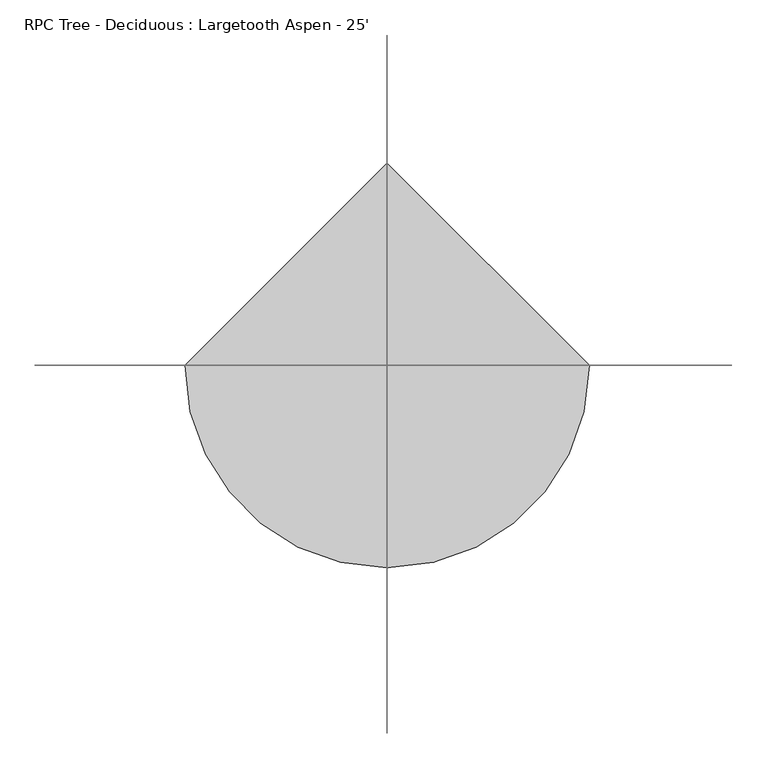
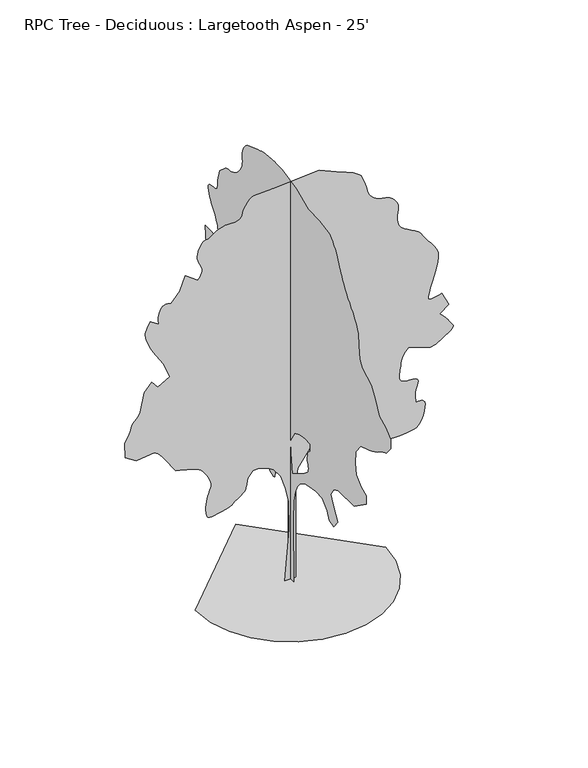
"""IFC4 building model written with IfcOpenShell, lengths in millimetres: geographic element geometry, RPC Tree - Deciduous : Largetooth Aspen - 25'."""

from ifc_helpers import new_model, si_unit, origin, place, context, project, spatial, triangles, source, transform, mapped, element, save


def rpc_tree_deciduous_largetooth_aspen_25_807f66b4(model_context):
    return source(origin(), model_context, "Body", "Tessellation", [
        triangles([(26.0697205, 0.000114, 0.0015477), (-29.1730399, 0.000114, 0.0015477), (-6.4261123, 9.81e-05, 266.4664568), (-9.6756528, 8.92e-05, 415.9470311), (-25.9234267, 8.45e-05, 493.9371471), (-48.6706393, 8.05e-05, 562.1781489), (-84.4157958, 7.76e-05, 610.9215763), (-113.6617395, 7.66e-05, 627.1696398), (-159.1557286, 7.56e-05, 643.4177032), (-191.6518556, 7.56e-05, 643.4177032), (-214.3988501, 7.76e-05, 610.9215763), (-224.1479643, 8.01e-05, 568.6770982), (-224.9530387, 8.04e-05, 563.7605742), (-226.4124337, 8.07e-05, 558.5873071), (-229.1782896, 8.1e-05, 552.903388), (-233.9063258, 8.14e-05, 546.4513836), (-241.248047, 8.18e-05, 538.9766945), (-251.8591362, 8.24e-05, 530.2225413), (-266.392497, 8.3e-05, 519.9336345), (-280.2623081, 8.36e-05, 510.0998597), (-289.8115798, 8.4e-05, 502.539093), (-297.0878617, 8.44e-05, 496.7414091), (-304.1365594, 8.46e-05, 492.1940123), (-313.003787, 8.49e-05, 488.3855238), (-325.7370941, 8.51e-05, 484.8039474), (-344.3818863, 8.53e-05, 480.9385583), (-364.9121012, 8.56e-05, 476.5525978), (-382.0882693, 8.58e-05, 472.5065875), (-396.1379931, 8.6e-05, 469.9398474), (-407.2889113, 8.6e-05, 469.9867922), (-415.7685173, 8.57e-05, 473.7860152), (-421.803069, 8.52e-05, 482.4733483), (-425.6214769, 8.43e-05, 497.1866218), (-427.2885263, 8.33e-05, 514.7041572), (-427.0232446, 8.23e-05, 531.0845163), (-425.2801097, 8.14e-05, 546.3852539), (-422.5135271, 8.05e-05, 560.6625801), (-419.1787379, 7.98e-05, 573.9733955), (-415.7301112, 7.9e-05, 586.3745645), (-412.6228881, 7.83e-05, 597.9237505), (-409.3641844, 7.77e-05, 608.0227707), (-405.6503122, 7.72e-05, 616.6439014), (-402.2209067, 7.67e-05, 624.6968256), (-399.8141859, 7.62e-05, 633.0910807), (-399.1698575, 7.57e-05, 642.7356955), (-401.0267936, 7.5e-05, 654.5402075), (-406.1239388, 7.41e-05, 669.4142269), (-413.6370704, 7.31e-05, 685.5008177), (-422.0590854, 7.22e-05, 700.2233202), (-431.1069706, 7.14e-05, 713.4111053), (-440.4954964, 7.08e-05, 724.8969595), (-449.9409591, 7.02e-05, 734.4981903), (-459.1587831, 6.97e-05, 742.058194), (-467.8659914, 6.94e-05, 747.406414), (-477.7374455, 6.92e-05, 751.5811592), (-490.3384933, 6.89e-05, 755.763026), (-505.2125127, 6.87e-05, 759.9377712), (-521.9057888, 6.84e-05, 764.1196381), (-539.9631168, 6.82e-05, 768.2943832), (-558.9300914, 6.79e-05, 772.4691284), (-578.351544, 6.77e-05, 776.6509953), (-633.5939569, 6.28e-05, 857.8912399), (-646.194932, 6.18e-05, 874.9245026), (-656.4077534, 6.11e-05, 887.526931), (-664.6306526, 6.05e-05, 896.4311113), (-671.2625879, 6.02e-05, 902.3767513), (-676.7004101, 6e-05, 906.110535), (-681.3431499, 5.98e-05, 908.3650486), (-685.5875856, 5.97e-05, 909.8799271), (-776.5727297, 6.03e-05, 900.1364811), (-831.8187035, 5.82e-05, 935.8813923), (-835.0688684, 5.37e-05, 1010.621307), (-828.8316765, 5.31e-05, 1021.7515869), (-822.8006493, 5.24e-05, 1032.8249662), (-817.1608772, 5.18e-05, 1043.791666), (-812.1184525, 5.11e-05, 1054.5805424), (-807.879685, 5.05e-05, 1065.1418163), (-804.62952, 4.99e-05, 1075.41866), (-802.5741949, 4.93e-05, 1085.3612217), (-799.3666872, 4.87e-05, 1094.7561424), (-793.2717104, 4.82e-05, 1103.6461521), (-785.3489382, 4.77e-05, 1112.3014378), (-776.6865309, 4.71e-05, 1121.0207457), (-768.3725761, 4.66e-05, 1130.0743355), (-761.473942, 4.6e-05, 1139.7608809), (-757.0787888, 4.54e-05, 1150.3506414), (-737.5776535, 3.96e-05, 1247.8418564), (-698.5861382, 3.71e-05, 1290.0799759), (-669.3395222, 3.92e-05, 1254.3350647), (-607.5974696, 3.73e-05, 1286.8368599), (-640.0935602, 3.24e-05, 1368.0701283), (-692.0865349, 2.76e-05, 1449.3103729), (-698.3393509, 2.69e-05, 1460.8602493), (-705.5018497, 2.6e-05, 1475.2548649), (-712.891951, 2.51e-05, 1491.3493767), (-719.8261208, 2.41e-05, 1508.0127491), (-725.6224239, 2.31e-05, 1524.1071156), (-729.6051023, 2.23e-05, 1538.5018764), (-731.0844452, 2.16e-05, 1550.0517529), (-730.3234451, 2.1e-05, 1559.7027626), (-728.2040977, 2.04e-05, 1569.1901196), (-724.9396894, 1.99e-05, 1578.5282124), (-720.7720659, 1.93e-05, 1587.7523586), (-715.9216352, 1.88e-05, 1596.8984573), (-710.6175259, 1.82e-05, 1605.9804611), (-705.0850874, 1.77e-05, 1615.0410999), (-662.8405729, 1.94e-05, 1585.796664), (-664.186203, 1.89e-05, 1594.8715462), (-665.2472574, 1.84e-05, 1604.0887161), (-665.7394512, 1.78e-05, 1613.5903164), (-665.3795895, 1.72e-05, 1623.5186348), (-663.8825151, 1.66e-05, 1634.0159592), (-660.964452, 1.59e-05, 1645.224432), (-656.3416237, 1.52e-05, 1657.2863411), (-650.2971525, 1.46e-05, 1667.8335171), (-643.3999718, 1.41e-05, 1674.7960281), (-635.7922239, 1.39e-05, 1678.7716576), (-627.6162695, 1.38e-05, 1680.3647289), (-619.0136696, 1.38e-05, 1680.1656132), (-610.1272207, 1.39e-05, 1678.7716576), (-601.0985204, 1.4e-05, 1676.7803547), (-558.8540059, 1.11e-05, 1725.5259258), (-529.6080803, 6.9e-06, 1797.0157482), (-467.8659914, 9.6e-06, 1751.5202694), (-461.6700397, 9.1e-06, 1759.8911247), (-455.9000793, 8.6e-06, 1768.3116863), (-450.982865, 8.1e-06, 1776.8460491), (-447.3450783, 7.5e-06, 1785.5511864), (-445.4127471, 7e-06, 1794.4909023), (-445.6111725, 6.5e-06, 1803.7080723), (-448.3684896, 5.9e-06, 1813.2666458), (-452.8589859, 5.3e-06, 1823.0455547), (-457.6339851, 4.7e-06, 1832.9881165), (-462.181382, 4.1e-06, 1843.2792034), (-465.9898705, 3.5e-06, 1854.0823231), (-468.5480355, 2.8e-06, 1865.5611282), (-469.3438808, 2e-06, 1877.8932243), (-467.8659914, 1.2e-06, 1891.2566528), (-464.322821, 4e-07, 1904.904657), (-459.4148357, -3e-07, 1917.7062012), (-453.3703282, -1e-06, 1929.1992496), (-446.4169373, -1.6e-06, 1938.9284523), (-438.7808118, -2e-06, 1946.4386044), (-430.6894815, -2.3e-06, 1951.2819134), (-422.3720023, -2.4e-06, 1952.9959076), (-413.0588717, -2.6e-06, 1955.3357357), (-401.9840753, -2.9e-06, 1961.3738846), (-389.3737985, -3.4e-06, 1969.6238171), (-375.456334, -4e-06, 1978.6133846), (-360.4592843, -4.5e-06, 1986.8631718), (-344.6094887, -4.8e-06, 1992.9013206), (-328.1338228, -5e-06, 1995.2411488), (-311.3459667, -5e-06, 1995.1487125), (-294.899496, -5e-06, 1995.276757), (-279.5326106, -5e-06, 1996.2652142), (-265.9849819, -5.2e-06, 1998.7259651), (-254.9948097, -5.4e-06, 2003.2919655), (-247.3017654, -5.9e-06, 2010.5889038), (-243.6447939, -6.5e-06, 2021.2354923), (-240.5752501, -7.3e-06, 2034.9474461), (-234.6068645, -8.2e-06, 2050.1315483), (-226.4216809, -9.1e-06, 2065.4934013), (-216.7009988, -1e-05, 2079.7102661), (-206.1283157, -1.07e-05, 2091.4877449), (-195.3849308, -1.12e-05, 2099.510075), (-185.1529063, -1.13e-05, 2102.475737), (-90.9154535, -1.17e-05, 2108.9762123), (143.0548945, -1.27e-05, 2125.2271099), (260.03936, -9.6e-06, 2073.2313011), (279.432326, -9.1e-06, 2065.5361313), (298.2008752, -8.7e-06, 2057.648822), (315.7177202, -8.2e-06, 2049.3563049), (331.359825, -7.7e-06, 2040.4734169), (344.499975, -7.1e-06, 2030.7869442), (354.5136443, -6.4e-06, 2020.1117237), (360.7764524, -5.7e-06, 2008.2418087), (364.9448027, -5e-06, 1996.5852528), (369.0562523, -4.4e-06, 1986.2444595), (373.0545911, -3.8e-06, 1976.5223785), (376.8823008, -3.3e-06, 1966.7434696), (380.4823717, -2.6e-06, 1956.2247803), (383.797976, -1.9e-06, 1944.2907703), (386.7729398, -1.1e-06, 1930.2518017), (391.2164912, -2e-07, 1915.7361179), (398.4451198, 5e-07, 1902.8706242), (407.6629801, 1.2e-06, 1891.7118576), (418.0749536, 1.8e-06, 1882.3098152), (428.8844682, 2.2e-06, 1874.7355682), (439.2964053, 2.6e-06, 1869.0317013), (448.5149923, 2.8e-06, 1865.2553329), (457.0415431, 2.9e-06, 1862.9936977), (465.7950059, 3e-06, 1861.4716976), (474.6060596, 3.1e-06, 1860.2271515), (483.3033122, 3.2e-06, 1858.8189526), (491.7160618, 3.3e-06, 1856.7777981), (499.674406, 3.5e-06, 1853.6627266), (507.0068436, 3.8e-06, 1849.0114117), (514.1032127, 4.1e-06, 1842.6889778), (521.1988552, 4.6e-06, 1835.0648792), (527.8969202, 5.1e-06, 1826.4167152), (533.7991762, 5.7e-06, 1817.0287708), (538.5080094, 6.3e-06, 1807.1859123), (541.6251884, 6.8e-06, 1797.172134), (542.7524451, 7.4e-06, 1787.2651806), (541.7674398, 8.1e-06, 1775.6939392), (539.645222, 9e-06, 1761.1000626), (537.6368053, 1e-05, 1744.4651768), (536.9924406, 1.1e-05, 1726.7492523), (538.9631779, 1.21e-05, 1708.9193813), (544.7992679, 1.31e-05, 1691.943092), (555.751034, 1.4e-05, 1676.7803547), (571.0795315, 1.48e-05, 1664.08549), (588.4548154, 1.54e-05, 1653.2111538), (606.7397458, 1.6e-05, 1643.1903992), (624.7971102, 1.66e-05, 1633.0487217), (641.49035, 1.73e-05, 1621.8331272), (655.6823616, 1.81e-05, 1608.5692566), (666.2365866, 1.91e-05, 1592.296994), (677.0367994, 2.01e-05, 1574.1543514), (691.3610704, 2.12e-05, 1555.7839611), (707.1639576, 2.24e-05, 1536.9585114), (722.4006729, 2.35e-05, 1517.4503998), (735.0173447, 2.47e-05, 1497.0318787), (742.9756525, 2.6e-05, 1475.4824673), (744.227393, 2.74e-05, 1452.5606106), (739.640173, 2.9e-05, 1426.0825756), (732.2152628, 3.08e-05, 1395.5081337), (723.0834074, 3.27e-05, 1363.1201397), (713.3755697, 3.46e-05, 1331.1802288), (704.2458944, 3.64e-05, 1301.9712559), (696.8181501, 3.78e-05, 1277.7690994), (692.2330376, 3.88e-05, 1260.8353947), (692.0054352, 3.94e-05, 1250.6723522), (696.3828569, 3.98e-05, 1244.7695148), (704.5965271, 3.99e-05, 1242.4224197), (715.878978, 3.99e-05, 1242.9132328), (729.4628872, 3.97e-05, 1245.5374912), (744.5829672, 3.95e-05, 1249.5841919), (760.4711689, 3.92e-05, 1254.3350647), (796.2160801, 4.35e-05, 1182.845315), (750.7277229, 4.56e-05, 1147.1004765), (757.676136, 4.6e-05, 1140.8134329), (764.5747702, 4.64e-05, 1134.3771252), (771.3596031, 4.68e-05, 1127.6633635), (777.973807, 4.72e-05, 1120.5158346), (784.3603357, 4.76e-05, 1112.8064215), (790.4624342, 4.81e-05, 1104.3857872), (796.2160801, 4.87e-05, 1095.1117893), (802.3750065, 4.92e-05, 1086.0795645), (808.8754091, 4.97e-05, 1078.1852062), (814.4654022, 5.01e-05, 1070.9807768), (817.8933907, 5.05e-05, 1063.9968281), (817.9147556, 5.1e-05, 1056.785277), (813.270635, 5.14e-05, 1048.8980404), (802.7164101, 5.2e-05, 1039.8658155), (731.2266603, 5.49e-05, 991.1202444), (701.9814251, 5.51e-05, 987.8700068), (594.7461102, 5.3e-05, 1023.6149179), (587.1284429, 5.34e-05, 1015.9055048), (579.7675186, 5.39e-05, 1007.8831747), (572.917973, 5.44e-05, 999.2350107), (566.8350958, 5.5e-05, 989.6409016), (561.7763203, 5.56e-05, 978.8093679), (557.9962821, 5.64e-05, 966.4060553), (555.751034, 5.72e-05, 952.1251682), (554.18783, 5.8e-05, 938.2638777), (552.3970236, 5.87e-05, 926.7922668), (550.5493166, 5.93e-05, 916.9136547), (548.8154108, 5.99e-05, 907.8245293), (547.366008, 6.04e-05, 898.7425255), (546.3710469, 6.1e-05, 888.8568644), (546.0019197, 6.17e-05, 877.3852535), (548.5217151, 6.23e-05, 866.5607689), (555.0213547, 6.28e-05, 858.8015768), (563.9077672, 6.31e-05, 853.5956446), (573.5900614, 6.33e-05, 850.4449648), (582.4764739, 6.34e-05, 848.8234795), (588.9761498, 6.34e-05, 848.2260595), (591.4959088, 6.34e-05, 848.140745), (595.0490713, 6.34e-05, 848.3896397), (604.0016499, 6.34e-05, 848.5176115), (615.7968601, 6.34e-05, 847.6286396), (627.8765734, 6.36e-05, 844.8051928), (637.6819342, 6.4e-05, 839.1440557), (642.6560492, 6.45e-05, 829.7206484), (640.2400629, 6.54e-05, 815.6459988), (634.4132383, 6.63e-05, 799.5017807), (630.6332365, 6.72e-05, 784.3817007), (628.5579271, 6.81e-05, 770.115057), (627.8474327, 6.89e-05, 756.5240261), (628.1603497, 6.97e-05, 743.4521496), (629.1553471, 7.04e-05, 730.7216766), (630.4909487, 7.12e-05, 718.1547838), (641.5372948, 7.11e-05, 719.3994026), (652.016161, 7.11e-05, 719.7336845), (661.3570152, 7.12e-05, 718.2401711), (668.993177, 7.14e-05, 714.0298903), (674.3556404, 7.19e-05, 706.1732477), (676.8753994, 7.26e-05, 693.7720425), (675.9849741, 7.37e-05, 675.9131035), (672.4133171, 7.49e-05, 655.5067183), (667.3069427, 7.6e-05, 636.4067213), (660.7226063, 7.71e-05, 619.1267441), (652.7166269, 7.8e-05, 604.1766028), (643.347286, 7.87e-05, 592.0684393), (632.6701035, 7.92e-05, 583.3149765), (620.7425611, 7.95e-05, 578.4262124), (609.5532732, 7.96e-05, 576.0102625), (600.0701311, 7.97e-05, 574.2194561), (590.8138647, 7.98e-05, 572.8838181), (580.3073112, 7.99e-05, 571.8319565), (567.0718909, 7.99e-05, 570.8945864), (549.630441, 8e-05, 569.8996253), (526.5043817, 8.01e-05, 568.6770982), (501.3699057, 8e-05, 569.0845951), (478.622893, 7.98e-05, 572.7323376), (457.865112, 7.95e-05, 579.0798062), (438.6997121, 7.89e-05, 587.5871721), (420.7277349, 7.83e-05, 597.7153693), (403.5515305, 7.77e-05, 608.9231518), (386.7729398, 7.7e-05, 620.6707632), (315.281773, 7.29e-05, 688.9117287), (240.541822, 7.1e-05, 721.4050215), (152.8033002, 7.14e-05, 714.9117405), (110.5587767, 7.33e-05, 682.4127794), (81.3128329, 7.58e-05, 640.168265), (35.8184146, 7.97e-05, 575.1767378), (26.0697205, 8.45e-05, 493.9371471), (26.0697205, 9.5e-05, 318.4601037), (-0.0006638, 25.4362563, 3.1e-06), (-0.0006638, -26.5568933, 0.0), (-0.0006638, -23.3073528, 324.9576359), (-0.0006638, -26.5568933, 428.9442029), (-0.0006638, -39.5552709, 484.1866158), (-0.0006638, -59.0527272, 526.4311303), (-0.0006638, -85.049478, 558.9272573), (-0.0006638, -124.044536, 581.67427), (-0.0006638, -156.5399363, 588.1731829), (-0.0006638, -221.5314634, 601.1717717), (-0.0006638, -276.7745849, 597.9222971), (-0.0006638, -319.0191175, 555.6777826), (-0.0006638, -338.5166556, 516.6827428), (-0.0006638, -374.2615305, 503.6841539), (-0.0006638, -413.2565703, 552.4276176), (-0.0006638, -371.0120559, 617.4198715), (-0.0006638, -351.5145178, 662.9138243), (-0.0006638, -374.2615305, 701.9081738), (-0.0006638, -416.506045, 721.4050215), (-0.0006638, -552.9880122, 721.4050215), (-0.0006638, -660.2240902, 796.1449362), (-0.0006638, -660.2240902, 841.6403423), (-0.0006638, -614.7300648, 861.1343559), (-0.0006638, -572.4855503, 900.1293594), (-0.0006638, -562.7371628, 955.3753332), (-0.0006638, -569.2360757, 1020.364753), (-0.0006638, -611.4806265, 1075.6107267), (-0.0006638, -686.2205412, 1101.6049976), (-0.0006638, -698.7362017, 1106.4980856), (-0.0006638, -711.1374069, 1111.4693665), (-0.0006638, -723.3110098, 1116.6113491), (-0.0006638, -735.1453892, 1122.0164698), (-0.0006638, -746.5245638, 1127.7557997), (-0.0006638, -757.3348051, 1133.9219204), (-0.0006638, -767.4622393, 1140.6000738), (-0.0006638, -777.2056852, 1147.185791), (-0.0006638, -786.9562529, 1153.0887737), (-0.0006638, -796.7067478, 1158.4227505), (-0.0006638, -806.4573154, 1163.3015951), (-0.0006638, -816.2007614, 1167.8390362), (-0.0006638, -825.951329, 1172.1488749), (-0.0006638, -835.701824, 1176.344985), (-0.0006638, -871.4467352, 1221.8403912), (-0.0006638, -871.4467352, 1267.3357246), (-0.0006638, -829.201494, 1306.3308735), (-0.0006638, -773.9626419, 1335.5753094), (-0.0006638, -738.2106091, 1403.8148941), (-0.0006638, -702.4693314, 1455.8107029), (-0.0006638, -624.479179, 1498.0559441), (-0.0006638, -601.7322026, 1533.8008553), (-0.0006638, -595.232563, 1605.2905323), (-0.0006638, -588.7336138, 1663.7795494), (-0.0006638, -581.7610016, 1678.3663044), (-0.0006638, -574.7315251, 1692.6898487), (-0.0006638, -567.5875208, 1706.5013603), (-0.0006638, -560.2735414, 1719.5447502), (-0.0006638, -552.7327226, 1731.5711964), (-0.0006638, -544.9066741, 1742.3102211), (-0.0006638, -536.7406754, 1751.5202694), (-0.0006638, -526.6124783, 1762.4087036), (-0.0006638, -513.8137319, 1777.3297405), (-0.0006638, -499.6495165, 1794.754113), (-0.0006638, -485.4297812, 1813.1386013), (-0.0006638, -472.4596427, 1830.9612053), (-0.0006638, -462.0476692, 1846.6787052), (-0.0006638, -455.5010848, 1858.7548576), (-0.0006638, -450.7737571, 1868.9036568), (-0.0006638, -445.1367828, 1879.8490643), (-0.0006638, -438.8739747, 1891.5838131), (-0.0006638, -432.2711801, 1904.1222919), (-0.0006638, -425.6108308, 1917.4501122), (-0.0006638, -419.1780112, 1931.5745407), (-0.0006638, -413.2565703, 1946.4955776), (-0.0006638, -406.7384362, 1961.4378342), (-0.0006638, -398.5148466, 1975.6974289), (-0.0006638, -388.8702682, 1989.3880177), (-0.0006638, -378.0892038, 2002.6234016), (-0.0006638, -366.4546669, 2015.517382), (-0.0006638, -354.2526501, 2028.1839054), (-0.0006638, -341.7660939, 2040.7366276), (-0.0006638, -250.7774072, 2056.9804035), (-0.0006638, -153.2904798, 2060.2304958), (-0.0006638, -49.3039627, 2105.7259747), (-0.0006638, 74.1795065, 2131.7203182), (-0.0006638, 90.8727781, 2132.40298), (-0.0006638, 107.452253, 2133.0004726), (-0.0006638, 123.8048613, 2133.4271908), (-0.0006638, 139.8153757, 2133.5978199), (-0.0006638, 155.3721478, 2133.4271908), (-0.0006638, 170.3599684, 2132.8298435), (-0.0006638, 184.6657449, 2131.7203182), (-0.0006638, 198.4217548, 2130.297876), (-0.0006638, 211.9501987, 2128.7119263), (-0.0006638, 225.4224323, 2126.7774513), (-0.0006638, 239.0084853, 2124.3309437), (-0.0006638, 252.8782783, 2121.2087505), (-0.0006638, 267.2025493, 2117.2259995), (-0.0006638, 282.1526723, 2112.2263046), (-0.0006638, 376.3908337, 2079.7316311), (-0.0006638, 384.7090396, 2072.7121468), (-0.0006638, 392.7996431, 2065.3441372), (-0.0006638, 400.4357686, 2057.3004421), (-0.0006638, 407.3891596, 2048.239658), (-0.0006638, 413.4336671, 2037.8064285), (-0.0006638, 418.3416524, 2025.6733028), (-0.0006638, 421.8848228, 2011.4849247), (-0.0006638, 423.1066958, 1997.9295021), (-0.0006638, 422.1116984, 1986.9912163), (-0.0006638, 420.2647182, 1977.2976219), (-0.0006638, 418.9283898, 1967.4902264), (-0.0006638, 419.4689092, 1956.210537), (-0.0006638, 423.248911, 1942.0789867), (-0.0006638, 431.6332466, 1923.7514717), (-0.0006638, 443.1155763, 1905.1322594), (-0.0006638, 455.053038, 1890.609454), (-0.0006638, 467.1036106, 1879.4934174), (-0.0006638, 478.9273075, 1871.1084641), (-0.0006638, 490.1827251, 1864.7716415), (-0.0006638, 500.5278422, 1859.8004333), (-0.0006638, 509.6233626, 1855.5047653), (-0.0006638, 517.979248, 1852.3896938), (-0.0006638, 526.3351333, 1850.8676937), (-0.0006638, 534.6910186, 1850.1351803), (-0.0006638, 543.0475943, 1849.4097885), (-0.0006638, 551.4034796, 1847.8806667), (-0.0006638, 559.7593649, 1844.7655952), (-0.0006638, 568.1152502, 1839.2609894), (-0.0006638, 616.8594406, 1797.0157482), (-0.0006638, 636.3562157, 1735.2764935), (-0.0006638, 635.7218067, 1725.5615341), (-0.0006638, 635.4565613, 1716.0811535), (-0.0006638, 635.9302242, 1707.0490013), (-0.0006638, 637.5126131, 1698.7066326), (-0.0006638, 640.5722374, 1691.2674065), (-0.0006638, 645.4802227, 1684.9661922), (-0.0006638, 652.6042791, 1680.0305923), (-0.0006638, 662.5141394, 1677.2070728), (-0.0006638, 674.5838968, 1676.1473991), (-0.0006638, 687.3926353, 1675.429129), (-0.0006638, 699.5199474, 1673.6296749), (-0.0006638, 709.5428822, 1669.3270306), (-0.0006638, 716.0425581, 1661.0984631), (-0.0006638, 717.5929722, 1647.5357735), (-0.0006638, 715.1606352, 1631.7685673), (-0.0006638, 710.8507965, 1617.7080883), (-0.0006638, 704.9763004, 1605.0700516), (-0.0006638, 697.852244, 1593.5700268), (-0.0006638, 689.7900908, 1582.9234383), (-0.0006638, 681.1020309, 1572.8457104), (-0.0006638, 672.1018536, 1563.0452911), (-0.0006638, 665.1668844, 1551.2109844), (-0.0006638, 658.4026897, 1539.4121407), (-0.0006638, 651.9791719, 1527.6631485), (-0.0006638, 646.0676868, 1515.9994709), (-0.0006638, 640.8374828, 1504.4495945), (-0.0006638, 636.4607878, 1493.0420059), (-0.0006638, 633.1067774, 1481.8050465), (-0.0006638, 631.3636425, 1471.2366508), (-0.0006638, 631.4966286, 1461.685199), (-0.0006638, 633.1920919, 1452.9873287), (-0.0006638, 636.1385691, 1444.9719749), (-0.0006638, 640.023143, 1437.4689445), (-0.0006638, 644.5328968, 1430.3071724), (-0.0006638, 649.3548409, 1423.3160294), (-0.0006638, 691.5993553, 1429.8163593), (-0.0006638, 743.5944374, 1429.8163593), (-0.0006638, 737.0940348, 1335.5753094), (-0.0006638, 678.6007301, 1234.8410511), (-0.0006638, 676.5076893, 1223.013866), (-0.0006638, 674.3855078, 1211.2790445), (-0.0006638, 672.206353, 1199.7078758), (-0.0006638, 669.9418837, 1188.3997725), (-0.0006638, 667.5636858, 1177.425951), (-0.0006638, 665.0438541, 1166.8789204), (-0.0006638, 662.3533934, 1156.8509714), (-0.0006638, 658.3266043, 1146.0123161), (-0.0006638, 652.4243483, 1133.4098877), (-0.0006638, 645.5555815, 1119.676569), (-0.0006638, 638.6306408, 1105.4241686), (-0.0006638, 632.557683, 1091.2926184), (-0.0006638, 628.2471176, 1077.8936543), (-0.0006638, 626.6078281, 1065.8601591), (-0.0006638, 627.9342007, 1055.1921329), (-0.0006638, 631.6480728, 1045.3776157), (-0.0006638, 637.3512131, 1036.274247), (-0.0006638, 644.6459713, 1027.7398842), (-0.0006638, 653.1348427, 1019.6251179), (-0.0006638, 662.419523, 1011.8019035), (-0.0006638, 672.1018536, 1004.1209044), (-0.0006638, 759.8382133, 1023.6149179), (-0.0006638, 764.6814497, 1009.7109701), (-0.0006638, 769.325643, 995.9137018), (-0.0006638, 773.5714594, 982.3511576), (-0.0006638, 777.2128069, 969.1228226), (-0.0006638, 780.0647404, 956.3496923), (-0.0006638, 781.9209497, 944.1454954), (-0.0006638, 782.5894409, 932.6311546), (-0.0006638, 778.8201216, 921.6574059), (-0.0006638, 769.1335762, 910.9111868), (-0.0006638, 755.9835068, 900.2289173), (-0.0006638, 741.8092993, 889.4257977), (-0.0006638, 729.057534, 878.3453693), (-0.0006638, 720.174646, 866.8026146), (-0.0006638, 717.5929722, 854.6410749), (-0.0006638, 719.9328003, 842.956105), (-0.0006638, 723.9795736, 832.8072332), (-0.0006638, 729.4486439, 823.9457102), (-0.0006638, 736.0486044, 816.1012035), (-0.0006638, 743.5090502, 809.0247459), (-0.0006638, 751.5313803, 802.4532721), (-0.0006638, 759.8382133, 796.1449362), (-0.0006638, 779.3392759, 731.1555164), (-0.0006638, 760.6276274, 730.5083176), (-0.0006638, 742.4564981, 730.18123), (-0.0006638, 725.3664076, 730.4727819), (-0.0006638, 709.8935148, 731.7031574), (-0.0006638, 696.5826994, 734.1852734), (-0.0006638, 685.9716465, 738.231974), (-0.0006638, 678.6007301, 744.156249), (-0.0006638, 671.5143894, 751.4958447), (-0.0006638, 661.6997995, 759.5181747), (-0.0006638, 649.6108572, 768.1094381), (-0.0006638, 635.7026218, 777.163028), (-0.0006638, 620.4303709, 786.550827), (-0.0006638, 604.2491275, 796.1663012), (-0.0006638, 587.612752, 805.8955038), (-0.0006638, 586.9214787, 795.4337151), (-0.0006638, 586.2579291, 784.8937334), (-0.0006638, 585.6520068, 774.176001), (-0.0006638, 585.1306724, 763.2021795), (-0.0006638, 584.7231754, 751.8940762), (-0.0006638, 584.4578937, 740.1522057), (-0.0006638, 584.3633137, 727.9053514), (-0.0006638, 583.918101, 715.1464645), (-0.0006638, 582.3925764, 702.6094391), (-0.0006638, 579.5029635, 691.3262615), (-0.0006638, 574.9647958, 682.3160557), (-0.0006638, 568.4942968, 676.6036863), (-0.0006638, 559.8070001, 675.2104574), (-0.0006638, 548.6177121, 679.161161), (-0.0006638, 535.9889408, 686.5035908), (-0.0006638, 523.1901944, 694.528101), (-0.0006638, 510.2485062, 703.1207451), (-0.0006638, 497.1930167, 712.1664865), (-0.0006638, 484.0529031, 721.5543583), (-0.0006638, 470.8558888, 731.1768814), (-0.0006638, 457.6297339, 740.9060841), (-0.0006638, 379.6403083, 763.6502626), (-0.0006638, 301.6501923, 737.6559191), (-0.0006638, 252.9067286, 679.161161), (-0.0006638, 259.1880494, 670.8429914), (-0.0006638, 265.5547029, 662.7524242), (-0.0006638, 272.0913315, 655.1162624), (-0.0006638, 278.8839947, 648.1628351), (-0.0006638, 286.0180432, 642.118364), (-0.0006638, 293.5780832, 637.2103786), (-0.0006638, 301.6501923, 633.6672083), (-0.0006638, 309.3432547, 630.2185816), (-0.0006638, 315.8421676, 625.5765684), (-0.0006638, 321.3468461, 619.9396305), (-0.0006638, 326.054989, 613.506811), (-0.0006638, 330.1671653, 606.4773345), (-0.0006638, 333.8810374, 599.0495539), (-0.0006638, 337.3957938, 591.4226575), (-0.0006638, 328.3194583, 589.3196609), (-0.0006638, 319.101598, 587.131277), (-0.0006638, 309.5985806, 584.7722277), (-0.0006638, 299.6702259, 582.157162), (-0.0006638, 289.1729197, 579.2014194), (-0.0006638, 277.9651372, 575.8189588), (-0.0006638, 265.9046089, 571.9251194), (-0.0006638, 253.8448072, 567.1792972), (-0.0006638, 242.6370247, 561.4093369), (-0.0006638, 232.1397185, 554.7873573), (-0.0006638, 222.2106553, 547.4826433), (-0.0006638, 212.7083283, 539.6665506), (-0.0006638, 203.490468, 531.5090907), (-0.0006638, 194.4141506, 523.1816557), (-0.0006638, 194.4141506, 477.6876666), (-0.0006638, 182.6473543, 470.1560769), (-0.0006638, 171.3072762, 463.3911555), (-0.0006638, 160.8192354, 458.1616782), (-0.0006638, 151.6106223, 455.234386), (-0.0006638, 144.1074647, 455.3766375), (-0.0006638, 138.7357814, 459.3557914), (-0.0006638, 135.9215636, 467.9392791), (-0.0006638, 134.5482372, 477.6684817), (-0.0006638, 133.2879943, 485.2953781), (-0.0006638, 132.2553266, 491.8988631), (-0.0006638, 131.5640443, 498.558522), (-0.0006638, 131.3272129, 506.3561202), (-0.0006638, 131.6586334, 516.3697895), (-0.0006638, 132.6720981, 529.6806049), (-0.0006638, 133.4963755, 544.2423978), (-0.0006638, 133.2972416, 557.439412), (-0.0006638, 132.2460885, 569.4999404), (-0.0006638, 130.5121827, 580.6508223), (-0.0006638, 128.2669255, 591.1196963), (-0.0006638, 125.6802919, 601.1340923), (-0.0006638, 122.9236833, 610.9201956), (-0.0006638, 67.6807117, 614.1696339), (-0.0006638, 38.4346316, 558.9272573), (-0.0006638, 22.1867158, 464.6890778), (-0.0006638, 22.1867158, 344.4551376), (-0.0006638, 22.1867158, 165.7286377), (-0.0006302, -13.5587302, 568.6756448), (-0.0006302, -0.5603383, 672.6622118), (-0.0006302, 2.6892152, 734.4057541), (-0.0006302, -36.3057282, 796.1449362), (-0.0006302, -78.5505378, 815.6459988), (-0.0006302, -127.2940016, 822.1392797), (-0.0006302, -172.7879997, 822.1392797), (-0.0006302, -172.7879997, 783.1513252), (-0.0006302, -150.0410052, 763.6502626), (-0.0006302, -143.542065, 718.1547838), (-0.0006302, -146.3079209, 715.3242153), (-0.0006302, -148.9606932, 712.2092165), (-0.0006302, -151.3858813, 708.5216509), (-0.0006302, -153.4704107, 703.9834831), (-0.0006302, -155.0997625, 698.3081028), (-0.0006302, -156.1608715, 691.2124603), (-0.0006302, -156.5399363, 682.410672), (-0.0006302, -155.5926285, 673.3251074), (-0.0006302, -152.9398471, 665.4335833), (-0.0006302, -148.8661041, 658.5364025), (-0.0006302, -143.6551486, 652.4350307), (-0.0006302, -137.5921738, 646.9310789), (-0.0006302, -130.9602385, 641.8246319), (-0.0006302, -124.044536, 636.9166466), (-479.3205975, 0.0, 0.0008755), (-466.6491325, -109.8283707, 0.0008689), (-430.5600563, -210.6885206, 0.0008629), (-373.944326, -299.6901375, 0.0008576), (-299.6901375, -373.944326, 0.0008532), (-210.6885206, -430.5600563, 0.0008498), (-109.8283707, -466.6491325, 0.0008477), (2.1e-05, -479.3205975, 0.0008469), (109.8283707, -466.6491325, 0.0008477), (210.6885206, -430.5600563, 0.0008498), (299.6901375, -373.944326, 0.0008532), (373.944326, -299.6901375, 0.0008576), (430.5600563, -210.6885206, 0.0008629), (466.6491325, -109.8283707, 0.0008689), (479.3205975, 4.19e-05, 0.0008755), (-6.3e-05, 479.3205975, 0.000904)], [[122, 123, 124], [87, 88, 89], [1, 2, 3], [329, 1, 3], [329, 3, 4], [328, 329, 4], [328, 4, 5], [105, 106, 107], [327, 328, 5], [327, 5, 6], [104, 105, 107], [238, 239, 240], [238, 240, 241], [237, 238, 241], [236, 237, 241], [103, 104, 107], [86, 87, 89], [235, 236, 241], [102, 103, 107], [101, 102, 107], [100, 101, 107], [99, 100, 107], [98, 99, 107], [97, 98, 107], [96, 97, 107], [327, 6, 7], [326, 327, 7], [95, 96, 107], [70, 71, 72], [69, 70, 72], [69, 72, 73], [69, 73, 74], [69, 74, 75], [69, 75, 76], [69, 76, 77], [69, 77, 78], [94, 95, 107], [234, 235, 241], [93, 94, 107], [69, 78, 79], [69, 79, 80], [69, 80, 81], [69, 81, 82], [69, 82, 83], [69, 83, 84], [69, 84, 85], [68, 69, 85], [325, 326, 7], [325, 7, 8], [67, 68, 85], [92, 93, 107], [91, 92, 107], [60, 61, 62], [67, 85, 86], [67, 86, 89], [67, 89, 90], [66, 67, 90], [65, 66, 90], [64, 65, 90], [63, 64, 90], [62, 63, 90], [60, 62, 90], [59, 60, 90], [58, 59, 90], [57, 58, 90], [56, 57, 90], [55, 56, 90], [54, 55, 90], [53, 54, 90], [284, 285, 286], [283, 284, 286], [282, 283, 286], [282, 286, 287], [281, 282, 287], [280, 281, 287], [279, 280, 287], [279, 287, 288], [278, 279, 288], [277, 278, 288], [277, 288, 289], [276, 277, 289], [275, 276, 289], [275, 289, 290], [52, 53, 90], [325, 8, 9], [121, 122, 124], [275, 290, 291], [30, 31, 32], [29, 30, 32], [29, 32, 33], [28, 29, 33], [28, 33, 34], [27, 28, 34], [27, 34, 35], [27, 35, 36], [26, 27, 36], [26, 36, 37], [26, 37, 38], [25, 26, 38], [25, 38, 39], [24, 25, 39], [23, 24, 39], [22, 23, 39], [21, 22, 39], [20, 21, 39], [20, 39, 40], [20, 40, 41], [20, 41, 42], [19, 20, 42], [19, 42, 43], [18, 19, 43], [18, 43, 44], [17, 18, 44], [16, 17, 44], [15, 16, 44], [14, 15, 44], [13, 14, 44], [12, 13, 44], [11, 12, 44], [11, 44, 45], [11, 45, 46], [10, 11, 46], [10, 46, 47], [10, 47, 48], [10, 48, 49], [10, 49, 50], [10, 50, 51], [252, 253, 254], [251, 252, 254], [251, 254, 255], [250, 251, 255], [249, 250, 255], [249, 255, 256], [248, 249, 256], [247, 248, 256], [246, 247, 256], [245, 246, 256], [245, 256, 257], [245, 257, 258], [244, 245, 258], [243, 244, 258], [242, 243, 258], [241, 242, 258], [234, 241, 258], [233, 234, 258], [274, 275, 291], [324, 325, 9], [51, 52, 90], [10, 51, 90], [9, 10, 90], [324, 9, 90], [323, 324, 90], [323, 90, 91], [323, 91, 107], [323, 107, 108], [323, 108, 109], [323, 109, 110], [323, 110, 111], [323, 111, 112], [323, 112, 113], [323, 113, 114], [323, 114, 115], [323, 115, 116], [323, 116, 117], [323, 117, 118], [323, 118, 119], [323, 119, 120], [323, 120, 121], [323, 121, 124], [323, 124, 125], [323, 125, 126], [323, 126, 127], [323, 127, 128], [323, 128, 129], [322, 323, 129], [322, 129, 130], [167, 168, 169], [274, 291, 292], [296, 297, 298], [296, 298, 299], [295, 296, 299], [294, 295, 299], [294, 299, 300], [293, 294, 300], [293, 300, 301], [293, 301, 302], [293, 302, 303], [293, 303, 304], [293, 304, 305], [293, 305, 306], [293, 306, 307], [293, 307, 308], [293, 308, 309], [293, 309, 310], [293, 310, 311], [293, 311, 312], [293, 312, 313], [293, 313, 314], [293, 314, 315], [293, 315, 316], [293, 316, 317], [293, 317, 318], [293, 318, 319], [292, 293, 319], [274, 292, 319], [274, 319, 320], [274, 320, 321], [274, 321, 322], [273, 274, 322], [273, 322, 130], [272, 273, 130], [271, 272, 130], [270, 271, 130], [269, 270, 130], [268, 269, 130], [267, 268, 130], [266, 267, 130], [265, 266, 130], [264, 265, 130], [263, 264, 130], [262, 263, 130], [261, 262, 130], [260, 261, 130], [259, 260, 130], [258, 259, 130], [233, 258, 130], [232, 233, 130], [231, 232, 130], [230, 231, 130], [229, 230, 130], [228, 229, 130], [227, 228, 130], [226, 227, 130], [225, 226, 130], [224, 225, 130], [223, 224, 130], [222, 223, 130], [221, 222, 130], [220, 221, 130], [219, 220, 130], [218, 219, 130], [217, 218, 130], [216, 217, 130], [215, 216, 130], [214, 215, 130], [213, 214, 130], [212, 213, 130], [211, 212, 130], [210, 211, 130], [209, 210, 130], [208, 209, 130], [207, 208, 130], [206, 207, 130], [205, 206, 130], [204, 205, 130], [203, 204, 130], [202, 203, 130], [201, 202, 130], [200, 201, 130], [199, 200, 130], [198, 199, 130], [197, 198, 130], [196, 197, 130], [195, 196, 130], [194, 195, 130], [193, 194, 130], [192, 193, 130], [191, 192, 130], [190, 191, 130], [189, 190, 130], [188, 189, 130], [187, 188, 130], [186, 187, 130], [185, 186, 130], [184, 185, 130], [183, 184, 130], [182, 183, 130], [181, 182, 130], [180, 181, 130], [179, 180, 130], [178, 179, 130], [177, 178, 130], [176, 177, 130], [175, 176, 130], [174, 175, 130], [173, 174, 130], [172, 173, 130], [171, 172, 130], [170, 171, 130], [169, 170, 130], [167, 169, 130], [167, 130, 131], [167, 131, 132], [167, 132, 133], [167, 133, 134], [167, 134, 135], [167, 135, 136], [164, 165, 166], [164, 166, 167], [163, 164, 167], [162, 163, 167], [161, 162, 167], [160, 161, 167], [159, 160, 167], [158, 159, 167], [143, 144, 145], [142, 143, 145], [141, 142, 145], [140, 141, 145], [140, 145, 146], [139, 140, 146], [138, 139, 146], [137, 138, 146], [136, 137, 146], [136, 146, 147], [136, 147, 148], [136, 148, 149], [136, 149, 150], [136, 150, 151], [136, 151, 152], [136, 152, 153], [136, 153, 154], [136, 154, 155], [136, 155, 156], [157, 158, 167], [157, 167, 136], [157, 136, 156], [634, 330, 635], [633, 634, 635], [632, 633, 635], [631, 632, 635], [540, 541, 542], [592, 593, 594], [494, 495, 496], [635, 330, 331], [635, 331, 332], [635, 332, 333], [635, 333, 334], [635, 334, 335], [658, 635, 335], [658, 335, 336], [658, 336, 337], [658, 337, 338], [540, 542, 543], [657, 658, 338], [631, 635, 636], [630, 631, 636], [518, 519, 520], [656, 657, 338], [656, 338, 339], [655, 656, 339], [654, 655, 339], [653, 654, 339], [540, 543, 544], [539, 540, 544], [518, 520, 521], [539, 544, 545], [538, 539, 545], [538, 545, 546], [538, 546, 547], [538, 547, 548], [537, 538, 548], [537, 548, 549], [536, 537, 549], [536, 549, 550], [536, 550, 551], [535, 536, 551], [535, 551, 552], [534, 535, 552], [493, 494, 496], [493, 496, 497], [343, 344, 345], [342, 343, 345], [341, 342, 345], [340, 341, 345], [340, 345, 346], [534, 552, 553], [533, 534, 553], [518, 521, 522], [350, 351, 352], [349, 350, 352], [349, 352, 353], [348, 349, 353], [533, 553, 554], [652, 653, 339], [518, 522, 523], [518, 523, 524], [533, 554, 555], [532, 533, 555], [518, 524, 525], [518, 525, 526], [518, 526, 527], [518, 527, 528], [518, 528, 529], [518, 529, 530], [518, 530, 531], [518, 531, 532], [518, 532, 555], [517, 518, 555], [516, 517, 555], [515, 516, 555], [607, 608, 609], [591, 592, 594], [591, 594, 595], [590, 591, 595], [590, 595, 596], [589, 590, 596], [588, 589, 596], [588, 596, 597], [587, 588, 597], [586, 587, 597], [586, 597, 598], [585, 586, 598], [585, 598, 599], [584, 585, 599], [584, 599, 600], [583, 584, 600], [583, 600, 601], [582, 583, 601], [514, 515, 555], [643, 644, 645], [630, 636, 637], [629, 630, 637], [581, 582, 601], [581, 601, 602], [348, 353, 354], [580, 581, 602], [580, 602, 603], [579, 580, 603], [651, 652, 339], [651, 339, 340], [651, 340, 346], [650, 651, 346], [649, 650, 346], [649, 346, 347], [648, 649, 347], [647, 648, 347], [646, 647, 347], [372, 373, 374], [371, 372, 374], [370, 371, 374], [369, 370, 374], [369, 374, 375], [368, 369, 375], [367, 368, 375], [366, 367, 375], [365, 366, 375], [364, 365, 375], [363, 364, 375], [362, 363, 375], [361, 362, 375], [360, 361, 375], [359, 360, 375], [358, 359, 375], [357, 358, 375], [356, 357, 375], [356, 375, 376], [356, 376, 377], [356, 377, 378], [645, 646, 347], [643, 645, 347], [642, 643, 347], [641, 642, 347], [641, 347, 348], [641, 348, 354], [641, 354, 355], [607, 609, 610], [513, 514, 555], [579, 603, 604], [607, 610, 611], [607, 611, 612], [607, 612, 613], [607, 613, 614], [607, 614, 615], [607, 615, 616], [607, 616, 617], [607, 617, 618], [607, 618, 619], [607, 619, 620], [607, 620, 621], [607, 621, 622], [607, 622, 623], [607, 623, 624], [606, 607, 624], [606, 624, 625], [605, 606, 625], [605, 625, 626], [604, 605, 626], [579, 604, 626], [579, 626, 627], [579, 627, 628], [579, 628, 629], [579, 629, 637], [578, 579, 637], [578, 637, 638], [355, 356, 378], [641, 355, 378], [641, 378, 379], [640, 641, 379], [639, 640, 379], [639, 379, 380], [639, 380, 381], [639, 381, 382], [639, 382, 383], [639, 383, 384], [639, 384, 385], [639, 385, 386], [639, 386, 387], [639, 387, 388], [639, 388, 389], [639, 389, 390], [639, 390, 391], [639, 391, 392], [639, 392, 393], [639, 393, 394], [639, 394, 395], [638, 639, 395], [578, 638, 395], [577, 578, 395], [577, 395, 396], [577, 396, 397], [577, 397, 398], [577, 398, 399], [577, 399, 400], [577, 400, 401], [577, 401, 402], [577, 402, 403], [577, 403, 404], [577, 404, 405], [577, 405, 406], [577, 406, 407], [577, 407, 408], [577, 408, 409], [577, 409, 410], [577, 410, 411], [577, 411, 412], [577, 412, 413], [577, 413, 414], [577, 414, 415], [577, 415, 416], [577, 416, 417], [577, 417, 418], [577, 418, 419], [577, 419, 420], [577, 420, 421], [577, 421, 422], [577, 422, 423], [577, 423, 424], [577, 424, 425], [577, 425, 426], [577, 426, 427], [577, 427, 428], [577, 428, 429], [577, 429, 430], [577, 430, 431], [577, 431, 432], [577, 432, 433], [577, 433, 434], [566, 567, 568], [566, 568, 569], [565, 566, 569], [564, 565, 569], [564, 569, 570], [563, 564, 570], [563, 570, 571], [562, 563, 571], [562, 571, 572], [561, 562, 572], [560, 561, 572], [560, 572, 573], [559, 560, 573], [559, 573, 574], [558, 559, 574], [558, 574, 575], [557, 558, 575], [556, 557, 575], [556, 575, 576], [555, 556, 576], [513, 555, 576], [513, 576, 577], [512, 513, 577], [511, 512, 577], [470, 471, 472], [469, 470, 472], [468, 469, 472], [468, 472, 473], [467, 468, 473], [467, 473, 474], [467, 474, 475], [466, 467, 475], [466, 475, 476], [466, 476, 477], [465, 466, 477], [465, 477, 478], [465, 478, 479], [464, 465, 479], [464, 479, 480], [464, 480, 481], [464, 481, 482], [463, 464, 482], [456, 457, 458], [456, 458, 459], [456, 459, 460], [510, 511, 577], [463, 482, 483], [455, 456, 460], [454, 455, 460], [453, 454, 460], [452, 453, 460], [451, 452, 460], [450, 451, 460], [450, 460, 461], [449, 450, 461], [449, 461, 462], [463, 483, 484], [492, 493, 497], [448, 449, 462], [447, 448, 462], [491, 492, 497], [462, 463, 484], [447, 462, 484], [447, 484, 485], [446, 447, 485], [446, 485, 486], [445, 446, 486], [445, 486, 487], [444, 445, 487], [444, 487, 488], [491, 497, 498], [509, 510, 577], [491, 498, 499], [491, 499, 500], [490, 491, 500], [490, 500, 501], [490, 501, 502], [490, 502, 503], [490, 503, 504], [490, 504, 505], [490, 505, 506], [490, 506, 507], [490, 507, 508], [490, 508, 509], [490, 509, 577], [489, 490, 577], [488, 489, 577], [444, 488, 577], [443, 444, 577], [442, 443, 577], [441, 442, 577], [440, 441, 577], [435, 436, 437], [434, 435, 437], [434, 437, 438], [434, 438, 439], [577, 434, 439], [440, 577, 439], [673, 674, 659], [672, 673, 659], [672, 659, 660], [671, 672, 660], [671, 660, 661], [671, 661, 662], [670, 671, 662], [669, 670, 662], [669, 662, 663], [669, 663, 664], [669, 664, 665], [669, 665, 666], [669, 666, 667], [669, 667, 668]], closed=False),
    ])


if __name__ == "__main__":
    model = new_model("IFC4")
    model_context = context("Model", 3, world=origin())
    ifc_project = project(units=[si_unit("LENGTHUNIT", "METRE", prefix="MILLI")], contexts=[model_context])
    site = spatial("IfcSite", under=ifc_project)
    building = spatial("IfcBuilding", under=site)
    placement = place(None, origin())
    rpc_tree_deciduous_largetooth_aspen_25_shape = rpc_tree_deciduous_largetooth_aspen_25_807f66b4(model_context)
    element("IfcGeographicElement", 1, ObjectType="RPC Tree - Deciduous : Largetooth Aspen - 25'", at=placement, inside=building, context=model_context, shape_type="MappedRepresentation", body=[
        mapped(rpc_tree_deciduous_largetooth_aspen_25_shape, transform((0.0, 0.0, 0.0), x_axis=(1.0, 0.0, 0.0), y_axis=(0.0, 1.0, 0.0), z_axis=(0.0, 0.0, 1.0))),
    ])
    save(model, "model.ifc")

# Revit data of these elements
# Type "RPC Tree - Deciduous : Largetooth Aspen - 25'"
#   built-in parameter 1005198 = "{2, 15},{39, RPC-16-G0VG-J3PX-MQ0P-J000-ST1L-LVER-AU},{1, 0},{1, 0},{2, 35},{1, 8},{5, Color},{1, 0},{1, 0},{3, 0.8},{3, 0.8},{3, 0.8},{1, 8},{7, BBoxMin},{1, 0},{1, 0},{1, 0},{1, 0},{1, 0},{1, 8},{7, BBoxMax},{1, 0},{1, 0},{1, 0},{1, 0},{1, 0},{2, 11},{9, RPCTypeId},{1, 0},{1, 0},{39, RPC-16-G0VG-J3PX-MQ0P-J000-ST1L-LVER-AU},{1, 6},{14, RPCPlantHeight},{1, 0},{1, 0},{2, 25},{2, 11},{7, keyword},{1, 0},{1, 0},{178, :Geometry:RPC:Largetooth Aspen:Populus grandidentata:similar in form and aspect to trembling aspen; range does not extend as far west:east:or north; usually found on drier sites.},{2, 11},{8, category},{1, 0},{1, 0},{16, :Trees [General]},{2, 11},{12, LocalizedUID},{1, 0},{1, 0},{16, Largetooth Aspen},{2, 14},{6, Height},{1, 0},{1, 0},{2, 25},{1, 2},{16, Cast Reflections},{1, 0},{1, 0},{1, 0},{1, 2},{12, Cast Shadows},{1, 0},{1, 0},{1, 1},{1, 2},{9, Lock View},{1, 0},{1, 0},{1, 0},{1, 4},{5, ViewC},{1, 0},{1, 0},{1, 0},{2, 11},{20, AdvancedUIDefinition},{1, 0},{1, 0},{0, },{2, 11},{10, AssetLibID},{1, 0},{1, 0},{36, 4D3F6E72-3F99-4203-98E9-AF80B3C7A7A4},{2, 11},{10, BaseSchema},{1, 0},{1, 0},{9, RPCSchema},{2, 11},{12, ExchangeGUID},{1, 0},{1, 0},{0, },{1, 2},{6, Hidden},{1, 0},{1, 0},{1, 0},{1, 4},{11, RPCCategory},{1, 0},{1, 0},{1, 0},{2, 11},{8, RPCImage},{1, 0},{1, 0},{0, },{1, 4},{13, SchemaVersion},{1, 0},{1, 0},{1, 4},{2, 11},{12, UIDefinition},{1, 0},{1, 0},{0, },{2, 11},{6, UIName},{1, 0},{1, 0},{39, RPC-16-G0VG-J3PX-MQ0P-J000-ST1L-LVER-AU},{2, 11},{11, VersionGUID},{1, 0},{1, 0},{9, RPCSchema},{2, 11},{9, assettype},{1, 0},{1, 0},{11, RPCGeometry},{2, 11},{11, description},{1, 0},{1, 0},{0, },{2, 11},{9, localname},{1, 0},{1, 0},{3, RPC},{2, 11},{9, localtype},{1, 0},{1, 0},{3, RPC},{1, 4},{8, revision},{1, 0},{1, 0},{1, 1},{2, 11},{9, thumbnail},{1, 0},{1, 0},{0, },{1, 4},{7, version},{1, 0},{1, 0},{1, 1},{1, 2},{20, RPC_Cast Reflections},{1, 0},{1, 0},{1, 1},{1, 2},{16, RPC_Cast Shadows},{1, 0},{1, 0},{1, 1},{1, 2},{13, RPC_Lock View},{1, 0},{1, 0},{1, 0},{1, 4},{9, RPC_ViewC},{1, 0},{1, 0},{1, 0},{21, assetlibrary_base.fbx},{1, 5},"
#   built-in parameter 1005195 = "RPC-16-G0VG-J3PX-MQ0P-J000-ST1L-LVER-AU"
#   Type Comments = "Largetooth Aspen"
#   Assembly Code = "G2050500"
#   Height = 7' - 0"
#   Default Elevation = 0
